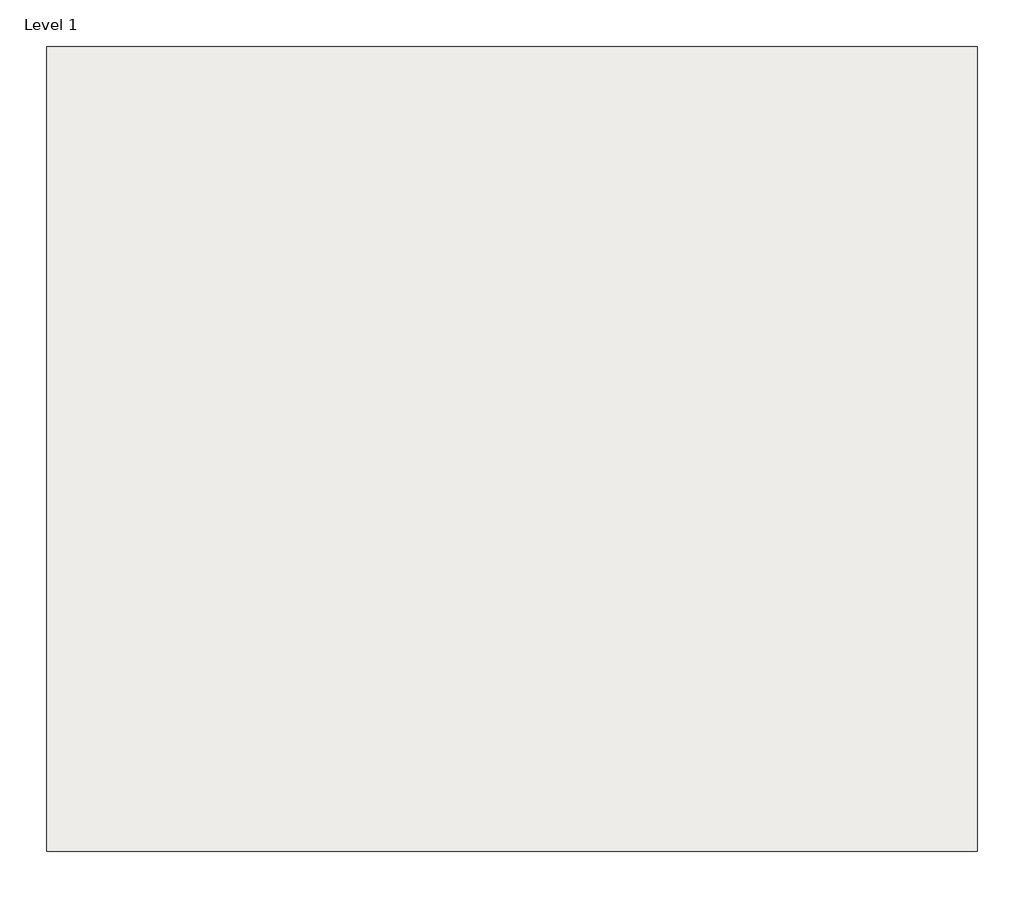
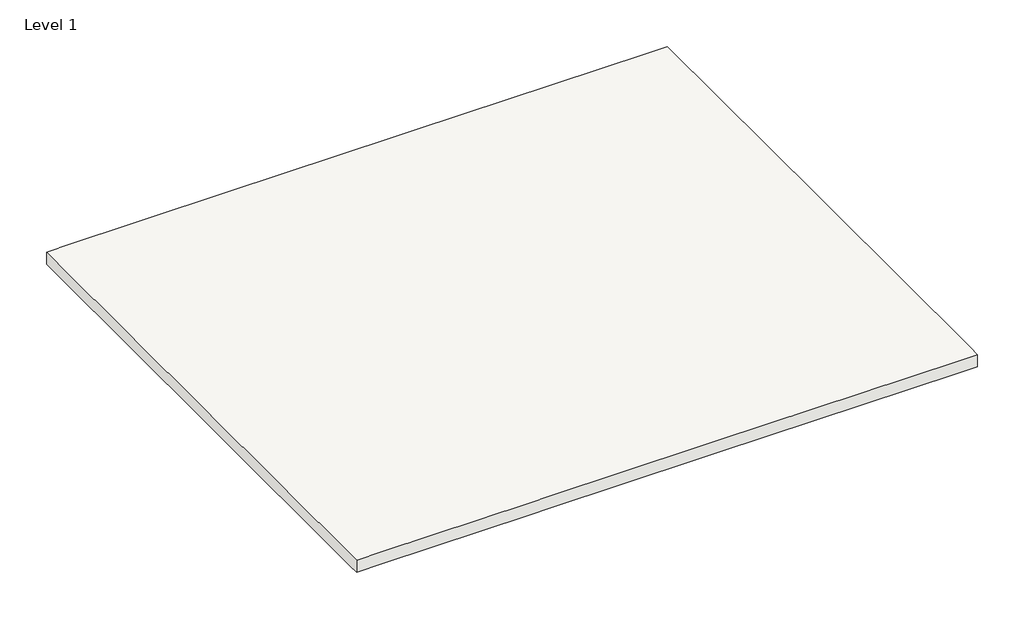
# One storey: 1 covering, 1 slab.
"""IFC4 building model written with IfcOpenShell, lengths in millimetres."""

from ifc_helpers import new_model, si_unit, frame, origin, place, context, project, spatial, polyline, outline, extrude, faceted_brep, element, save

model = new_model("IFC4")

# Units and contexts
model_context = context("Model", 3, world=origin())
ifc_project = project(units=[si_unit("LENGTHUNIT", "METRE", prefix="MILLI")], contexts=[model_context])

# Site, building, storey
site = spatial("IfcSite", under=ifc_project)
building = spatial("IfcBuilding", under=site)
storey = spatial("IfcBuildingStorey", under=building, Name="Level 1", Elevation=3000.0)

# Covering
placement = place(None, origin())
element("IfcCovering", 1, ObjectType="Plain", at=placement, inside=storey, context=model_context, shape_type="SweptSolid", body=[
    extrude(outline(polyline([(827.2403741, 8026.4804551), (827.2403741, -1270.5438109), (-10023.2536634, -1270.5438109), (-10023.2536634, 8026.4804551), (827.2403741, 8026.4804551)])), frame((0.0, 0.0, 2600.1024), z_axis=(0.0, 0.0, 1.0), x_axis=(1.0, 0.0, 0.0)), (0.0, 0.0, 1.0), 57.0),
])

# Slab
element("IfcSlab", 2, ObjectType="SLAB", at=placement, inside=storey, context=model_context, shape_type="Brep", body=[
    faceted_brep([(1025.0682817, 8254.493892, 2769.876), (1025.0682817, 3492.195999, 2769.876), (1025.0682817, 3136.494399, 2769.876), (1025.0682817, 3136.1864821, 2769.876), (1025.0682817, -1270.5438109, 2769.876), (1025.0682817, -1501.447153, 2769.876), (669.6714817, -1501.447153, 2769.876), (-3680.0785183, -1501.447153, 2769.876), (-4036.4886614, -1501.447153, 2769.876), (-6754.2886614, -1501.447153, 2769.876), (-7102.1088358, -1501.447153, 2769.876), (-9794.5088358, -1501.447153, 2769.876), (-10252.3493191, -1501.447153, 2769.876), (-10252.3493191, -1290.9249414, 2769.876), (-10252.3493191, 3098.5198031, 2769.876), (-10252.3493191, 3271.6004551, 2769.876), (-10252.3493191, 7899.022462, 2769.876), (-10252.3493191, 7900.9118098, 2769.876), (-10252.3493191, 8254.493892, 2769.876), (-10027.7206387, 8254.493892, 2769.876), (-10023.2536634, 8254.493892, 2769.876), (-6975.3482492, 8254.493892, 2769.876), (-6747.0434356, 8254.493892, 2769.876), (-3746.8074298, 8254.493892, 2769.876), (-3575.083968, 8254.493892, 2769.876), (-3572.0383998, 8254.493892, 2769.876), (644.3616002, 8254.493892, 2769.876), (665.5777613, 8254.493892, 2769.876), (1021.2793613, 8254.493892, 2769.876), (1025.0682817, 8254.493892, 3000.0), (1021.2793613, 8254.493892, 3000.0), (665.5777613, 8254.493892, 3000.0), (-3575.083968, 8254.493892, 3000.0), (-3930.785568, 8254.493892, 3000.0), (-6975.3482492, 8254.493892, 3000.0), (-10023.2536634, 8254.493892, 3000.0), (-10027.7206387, 8254.493892, 3000.0), (-10252.3493191, 8254.493892, 3000.0), (-10252.3493191, 7900.9118098, 3000.0), (-10252.3493191, 7899.022462, 3000.0), (-10252.3493191, 3271.6004551, 3000.0), (-10252.3493191, -1501.447153, 3000.0), (-9794.5088358, -1501.447153, 3000.0), (-7102.1088358, -1501.447153, 3000.0), (-6754.2886614, -1501.447153, 3000.0), (-4036.4886614, -1501.447153, 3000.0), (-3680.0785183, -1501.447153, 3000.0), (669.6714817, -1501.447153, 3000.0), (1025.0682817, -1501.447153, 3000.0), (1025.0682817, -1270.5438109, 3000.0), (1025.0682817, 3136.1864821, 3000.0), (1025.0682817, 3136.494399, 3000.0), (1025.0682817, 3492.195999, 3000.0)], [[[0, 1, 2, 3, 4, 5, 6, 7, 8, 9, 10, 11, 12, 13, 14, 15, 16, 17, 18, 19, 20, 21, 22, 23, 24, 25, 26, 27, 28]], [[29, 30, 31, 32, 33, 34, 35, 36, 37, 38, 39, 40, 41, 42, 43, 44, 45, 46, 47, 48, 49, 50, 51, 52]], [[5, 4, 3, 2, 1, 0, 29, 52, 51, 50, 49, 48]], [[12, 11, 10, 9, 8, 7, 6, 5, 48, 47, 46, 45, 44, 43, 42, 41]], [[18, 17, 16, 15, 14, 13, 12, 41, 40, 39, 38, 37]], [[0, 28, 27, 26, 25, 24, 23, 22, 21, 20, 19, 18, 37, 36, 35, 34, 33, 32, 31, 30, 29]]]),
])

save(model, "model.ifc")

# Revit data of these elements
# Type "Plain"
#   Keynote = "K40"
#   built-in parameter 1002203 = 1 (stored number, unit not read)
#   built-in parameter 1002202 = 1 (stored number, unit not read)
#   Layers, outside or top first: 0.147638 ft "Metal Stud Layer" (function 1); 0.03937 ft "Gypsum Wall Board" (function 1)
# Type "SLAB"
#   Layers, outside or top first: 0.755 ft "Concrete, Cast-in-Place, Gray" (function 1)
# Element 1 (IfcCovering, "Plain")
#   Height Offset From Level = -1.312 ft
#   Phase Created = New Construction
#   Materials on its faces: "Gypsum Wall Board", "Metal Stud Layer"
# Element 2 (IfcSlab, "SLAB")
#   Height Offset From Level = 0.0 ft
#   built-in parameter 1001954 = 1
#   Phase Created = New Construction
#   Materials on its faces: "Concrete, Cast-in-Place, Gray"
# Materials
#   "Metal Stud Layer": class "Metal", colour RGB 127 127 127, transparency 0, Description = "Light gauge steel framing, thermal air layer", Cost = 0
#   "Gypsum Wall Board": class "Generic", colour RGB 249 249 249, transparency 0, Description = "Gypsum Wall Board", Cost = 0
#   "Concrete, Cast-in-Place, Gray": class "Concrete", colour RGB 192 192 192, transparency 0, Description = "Cast-in-place concrete", Cost = 0
